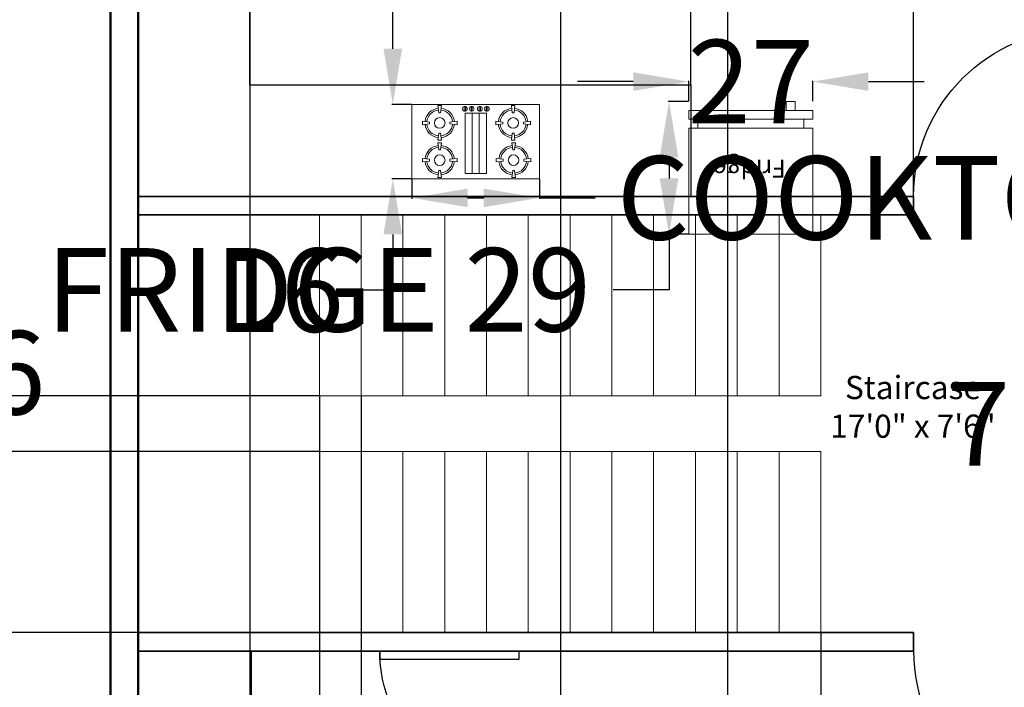
# Model space of a CAD drawing. Units: inches. Extents: x -230 to 384, y -962 to -183.
# Tile 3 of 6: x -121 to 91, y -640 to -496. Entities that reach past the tile are written whole.
import ezdxf

# ---------------------------------------------------------------- set-up
doc = ezdxf.new("R2010")
doc.units = ezdxf.units.IN
for name, color, linetype, lineweight in [('A-ANNO-DIMS', 2, 'Continuous', 18), ('A-ANNO-TEXT', 7, 'Continuous', 18), ('A-AREA-IDEN', 7, 'Continuous', 18), ('A-DOOR', 3, 'Continuous', 25), ('A-EQPM', 4, 'Continuous', 18), ('A-FLOR-STRS', 7, 'Continuous', 18), ('Inner Wall', 5, 'Continuous', 35), ('Kitchen', 4, 'Continuous', 25), ('Outer Wall', 1, 'Continuous', 50)]:
    doc.layers.add(name, color=color, linetype=linetype, lineweight=lineweight)
doc.styles.get("Standard").update_dxf_attribs({"font": 'arial.ttf'})
doc.dimstyles.get("Standard").update_dxf_attribs({"dimtxt": 18, "dimasz": 12, "dimexe": 0.18, "dimexo": 0.0625, "dimgap": 0.09, "dimtad": 0, "dimtih": 1, "dimtoh": 1, "dimdec": 0, "dimzin": 0, "dimdsep": 46, "dimlunit": 3, "dimtxsty": 'Standard', "dimcen": 0.09, "dimadec": 0, "dimazin": 0, "dimtfac": 1, "dimtdec": 0, "dimtofl": 0, "dimtmove": 0, "dimatfit": 3, "dimfxl": 1, "dimtolj": 1, "dimtzin": 0, "dimarcsym": 0})

# ---------------------------------------------------------------- blocks, each defined once
blk = doc.blocks.new('*U4')
for p, q in [((0, 0), (0, -4)), ((36, 0), (36, -4))]:
    blk.add_line(p, q)
blk.add_lwpolyline([(0, 0), (0, 36), (1.75, 36), (1.75, 0)], close=True)
blk.add_arc((0, 0), 36, 0, 90)
blk = doc.blocks.new('*U6')
for p, q in [((0, 0), (0, -4)), ((30, 0), (30, -4))]:
    blk.add_line(p, q)
blk.add_lwpolyline([(0, 0), (0, 30), (1.75, 30), (1.75, 0)], close=True)
blk.add_arc((0, 0), 30, 0, 90)
blk = doc.blocks.new('A$C57CF26DA')
for p, q in [((0, 0), (0, 420)), ((720, 420), (0, 420)), ((166.9, 413), (146.9, 413)), ((146.9, 413), (151.9, 373)), ((161.9, 373), (166.9, 413)), ((300, 390.9), (300, 49.1)), ((300, 390.9), (420, 390.9)), ((340, 390.9), (340, 49.1)), ((380, 390.9), (380, 49.1)), ((420, 390.9), (420, 49.1)), ((583.6, 413), (563.6, 413)), ((563.6, 413), (568.6, 373)), ((578.6, 373), (583.6, 413)), ((720, 0), (720, 420)), ((151.9, 373), (161.9, 373)), ((568.6, 373), (578.6, 373)), ((98.9, 320), (58.9, 325)), ((58.9, 325), (58.9, 305)), ((58.9, 305), (98.9, 310)), ((98.9, 310), (98.9, 320)), ((254.8, 325), (214.8, 320)), ((214.8, 320), (214.8, 310)), ((214.8, 310), (254.8, 305)), ((254.8, 305), (254.8, 325)), ((515.6, 320), (475.6, 325)), ((475.6, 325), (475.6, 305)), ((475.6, 305), (515.6, 310)), ((515.6, 310), (515.6, 320)), ((671.6, 325), (631.6, 320)), ((631.6, 320), (631.6, 310)), ((631.6, 310), (671.6, 305)), ((671.6, 305), (671.6, 325)), ((151.9, 257), (146.9, 217)), ((161.9, 257), (151.9, 257)), ((166.9, 217), (161.9, 257)), ((568.6, 257), (563.6, 217)), ((578.6, 257), (568.6, 257)), ((583.6, 217), (578.6, 257)), ((146.9, 217), (166.9, 217)), ((166.9, 203), (146.9, 203)), ((146.9, 203), (151.9, 163)), ((161.9, 163), (166.9, 203)), ((581.1, 203), (561.1, 203)), ((561.1, 203), (566.1, 163)), ((563.6, 217), (583.6, 217)), ((576.1, 163), (581.1, 203)), ((98.9, 110), (58.9, 115)), ((58.9, 115), (58.9, 95)), ((151.9, 163), (161.9, 163)), ((254.8, 115), (214.8, 110)), ((254.8, 95), (254.8, 115)), ((513.1, 110), (473.1, 115)), ((473.1, 115), (473.1, 95)), ((566.1, 163), (576.1, 163)), ((669, 115), (629, 110)), ((669, 95), (669, 115)), ((58.9, 95), (98.9, 100)), ((98.9, 100), (98.9, 110)), ((214.8, 110), (214.8, 100)), ((214.8, 100), (254.8, 95)), ((473.1, 95), (513.1, 100)), ((513.1, 100), (513.1, 110)), ((629, 110), (629, 100)), ((629, 100), (669, 95)), ((151.9, 47), (146.9, 7)), ((146.9, 7), (166.9, 7)), ((161.9, 47), (151.9, 47)), ((166.9, 7), (161.9, 47)), ((301.5, 38.7), (294.7, 38.7)), ((294.7, 38.7), (294.7, 11.3)), ((294.7, 11.3), (301.5, 11.3)), ((420, 49.1), (300, 49.1)), ((301.5, 11.3), (301.5, 38.7)), ((340.5, 38.7), (333.7, 38.7)), ((333.7, 38.7), (333.7, 11.3)), ((333.7, 11.3), (340.5, 11.3)), ((340.5, 11.3), (340.5, 38.7)), ((379.7, 11.3), (379.7, 38.7)), ((379.7, 38.7), (386.5, 38.7)), ((386.5, 11.3), (379.7, 11.3)), ((386.5, 38.7), (386.5, 11.3)), ((418.7, 11.3), (418.7, 38.7)), ((418.7, 38.7), (425.5, 38.7)), ((425.5, 11.3), (418.7, 11.3)), ((425.5, 38.7), (425.5, 11.3)), ((566.1, 47), (561.1, 7)), ((561.1, 7), (581.1, 7)), ((576.1, 47), (566.1, 47)), ((581.1, 7), (576.1, 47)), ((720, 0), (0, 0))]:
    blk.add_line(p, q)
for centre in [(156.9, 315), (573.6, 315), (156.9, 105), (571.1, 105)]:
    blk.add_circle(centre, 30)
for centre, radius, start, end in [((156.9, 315), 83, 95.5849, 174.4151), ((156.9, 315), 83, 5.5849, 84.4151), ((573.6, 315), 83, 95.5849, 174.4151), ((573.6, 315), 83, 5.5849, 84.4151), ((156.9, 315), 73, 95.3738, 174.6262), ((156.9, 315), 73, 5.3738, 84.6262), ((573.6, 315), 73, 95.3738, 174.6262), ((573.6, 315), 73, 5.3738, 84.6262), ((156.9, 315), 83, 185.5849, 264.4151), ((156.9, 315), 73, 185.3738, 264.6262), ((156.9, 315), 73, 275.3738, 354.6262), ((156.9, 315), 83, 275.5849, 354.4151), ((573.6, 315), 83, 185.5849, 264.4151), ((573.6, 315), 73, 185.3738, 264.6262), ((573.6, 315), 73, 275.3738, 354.6262), ((573.6, 315), 83, 275.5849, 354.4151), ((156.9, 105), 83, 95.5849, 174.4151), ((156.9, 105), 73, 95.3738, 174.6262), ((156.9, 105), 73, 5.3738, 84.6262), ((156.9, 105), 83, 5.5849, 84.4151), ((571.1, 105), 83, 95.5849, 174.4151), ((571.1, 105), 73, 95.3738, 174.6262), ((571.1, 105), 73, 5.3738, 84.6262), ((571.1, 105), 83, 5.5849, 84.4151), ((156.9, 105), 83, 185.5849, 264.4151), ((156.9, 105), 73, 185.3738, 264.6262), ((156.9, 105), 73, 275.3738, 354.6262), ((156.9, 105), 83, 275.5849, 354.4151), ((571.1, 105), 83, 185.5849, 264.4151), ((571.1, 105), 73, 185.3738, 264.6262), ((571.1, 105), 73, 275.3738, 354.6262), ((571.1, 105), 83, 275.5849, 354.4151), ((298.1, 25), 13.7, 104.4775, 255.5225), ((298.1, 25), 13.7, 284.4775, 75.5225), ((337.1, 25), 13.7, 104.4775, 255.5225), ((337.1, 25), 13.7, 284.4775, 75.5225), ((383.1, 25), 13.7, 104.4775, 255.5225), ((383.1, 25), 13.7, 284.4775, 75.5225), ((422.1, 25), 13.7, 104.4775, 255.5225), ((422.1, 25), 13.7, 284.4775, 75.5225)]:
    blk.add_arc(centre, radius, start, end)
blk = doc.blocks.new('REFRI-00')
for points in [[(-0.35, 0.35), (-0.35, -0.25), (0.35, -0.25), (0.35, 0.35), (-0.35, 0.35)], [(-0.3, -0.3), (-0.3, -0.25)], [(0.3, -0.3), (0.3, -0.25)], [(-0.35, -0.3), (-0.35, -0.35), (0.35, -0.35), (0.35, -0.3), (-0.35, -0.3)], [(-0.25, -0.35), (-0.25, -0.4), (-0.2, -0.4), (-0.2, -0.35)]]:
    blk.add_lwpolyline(points)
blk = doc.blocks.new('*D21')
at = {"layer": 'A-ANNO-DIMS', "color": 0, "lineweight": -2, "transparency": 16777216}
for p, q in [((-24.45, -424.96), (-24.45, -412.96)), ((-26.91, -436.96), (-24.27, -436.96)), ((-26.91, -450.25), (-24.27, -450.25)), ((-24.45, -462.25), (-24.45, -474.25)), ((-24.45, -474.25), (-36.45, -474.25))]:
    blk.add_line(p, q, dxfattribs=at)
at = {"layer": 'A-ANNO-DIMS', "color": 0, "transparency": 16777216}
for points in [[(-26.45, -424.96), (-22.45, -424.96), (-24.45, -436.96)], [(-26.45, -462.25), (-22.45, -462.25), (-24.45, -450.25)]]:
    blk.add_solid(points, dxfattribs=at)
at = {"layer": 'Defpoints', "color": 0, "transparency": 16777216}
for p in [(-26.97, -436.96), (-26.97, -450.25), (-24.45, -450.25)]:
    blk.add_point(p, dxfattribs=at)
at = {"layer": 'A-ANNO-DIMS', "color": 0, "transparency": 16777216, "insert": (-79.51, -474.25), "char_height": 18, "attachment_point": 5}
blk.add_mtext('\\A1;13 TYP.', dxfattribs=at)
blk = doc.blocks.new('*D23')
at = {"layer": 'A-ANNO-DIMS', "color": 0, "lineweight": -2, "transparency": 16777216}
for p, q in [((175.8, -568.08), (175.8, -583.43)), ((253.63, -568.08), (253.63, -583.43)), ((175.8, -583.25), (163.8, -583.25)), ((241.63, -583.25), (187.8, -583.25))]:
    blk.add_line(p, q, dxfattribs=at)
at = {"layer": 'A-ANNO-DIMS', "color": 0, "transparency": 16777216}
for points in [[(187.8, -581.25), (187.8, -585.25), (175.8, -583.25)], [(241.63, -581.25), (241.63, -585.25), (253.63, -583.25)]]:
    blk.add_solid(points, dxfattribs=at)
at = {"layer": 'Defpoints', "color": 0, "transparency": 16777216}
for p in [(175.8, -568.02), (253.63, -568.02), (175.8, -583.25)]:
    blk.add_point(p, dxfattribs=at)
at = {"layer": 'A-ANNO-DIMS', "color": 0, "transparency": 16777216, "insert": (119.97, -583.25), "char_height": 18, "attachment_point": 5}
blk.add_mtext('\\A1;78 TYP.', dxfattribs=at)
blk = doc.blocks.new('*D24')
at = {"layer": 'A-ANNO-DIMS', "color": 0, "lineweight": -2, "transparency": 16777216}
for p, q in [((14.93, -465.69), (14.93, -476.78)), ((88.09, -465.69), (88.09, -476.78)), ((26.93, -476.6), (76.09, -476.6)), ((88.09, -476.6), (100.09, -476.6))]:
    blk.add_line(p, q, dxfattribs=at)
at = {"layer": 'A-ANNO-DIMS', "color": 0, "transparency": 16777216}
for points in [[(26.93, -474.6), (26.93, -478.6), (14.93, -476.6)], [(76.09, -474.6), (76.09, -478.6), (88.09, -476.6)]]:
    blk.add_solid(points, dxfattribs=at)
at = {"layer": 'Defpoints', "color": 0, "transparency": 16777216}
for p in [(14.93, -465.63), (88.09, -465.63), (88.09, -476.6)]:
    blk.add_point(p, dxfattribs=at)
at = {"layer": 'A-ANNO-DIMS', "color": 0, "transparency": 16777216, "insert": (218.98, -476.6), "char_height": 18, "attachment_point": 5}
blk.add_mtext('\\A1;DINING SET 73 TYP.', dxfattribs=at)
blk = doc.blocks.new('*D28')
at = {"layer": 'A-ANNO-DIMS', "color": 0, "lineweight": -2, "transparency": 16777216}
for p, q in [((-36.67, -530.52), (-36.67, -534.76)), ((-9.19, -530.52), (-9.19, -534.76)), ((-24.67, -534.58), (-21.19, -534.58)), ((-9.19, -534.58), (2.81, -534.58))]:
    blk.add_line(p, q, dxfattribs=at)
at = {"layer": 'A-ANNO-DIMS', "color": 0, "transparency": 16777216}
for points in [[(-24.67, -532.58), (-24.67, -536.58), (-36.67, -534.58)], [(-21.19, -532.58), (-21.19, -536.58), (-9.19, -534.58)]]:
    blk.add_solid(points, dxfattribs=at)
at = {"layer": 'Defpoints', "color": 0, "transparency": 16777216}
for p in [(-36.67, -530.46), (-9.19, -530.46), (-9.19, -534.58)]:
    blk.add_point(p, dxfattribs=at)
at = {"layer": 'A-ANNO-DIMS', "color": 0, "transparency": 16777216, "insert": (82.05, -534.58), "char_height": 18, "attachment_point": 5}
blk.add_mtext('\\A1;COOKTOP 27', dxfattribs=at)
blk = doc.blocks.new('*D29')
at = {"layer": 'A-ANNO-DIMS', "color": 0, "lineweight": -2, "transparency": 16777216}
for p, q in [((-40.79, -502.43), (-40.79, -490.43)), ((-36.73, -514.43), (-40.97, -514.43)), ((-36.73, -530.46), (-40.97, -530.46)), ((-40.79, -542.46), (-40.79, -554.46)), ((-40.79, -554.46), (-52.79, -554.46))]:
    blk.add_line(p, q, dxfattribs=at)
at = {"layer": 'A-ANNO-DIMS', "color": 0, "transparency": 16777216}
for points in [[(-42.79, -502.43), (-38.79, -502.43), (-40.79, -514.43)], [(-42.79, -542.46), (-38.79, -542.46), (-40.79, -530.46)]]:
    blk.add_solid(points, dxfattribs=at)
at = {"layer": 'Defpoints', "color": 0, "transparency": 16777216}
for p in [(-36.67, -514.43), (-40.79, -530.46), (-36.67, -530.46)]:
    blk.add_point(p, dxfattribs=at)
at = {"layer": 'A-ANNO-DIMS', "color": 0, "transparency": 16777216, "insert": (-64.92, -554.46), "char_height": 18, "attachment_point": 5}
blk.add_mtext('\\A1;16', dxfattribs=at)
blk = doc.blocks.new('*D30')
at = {"layer": 'A-ANNO-DIMS', "color": 0, "lineweight": -2, "transparency": 16777216}
for p, q in [((22.93, -513.82), (18.53, -513.82)), ((18.71, -525.82), (18.71, -530.39)), ((22.93, -542.39), (18.53, -542.39)), ((18.71, -542.39), (18.71, -554.39)), ((18.71, -554.39), (6.71, -554.39))]:
    blk.add_line(p, q, dxfattribs=at)
at = {"layer": 'A-ANNO-DIMS', "color": 0, "transparency": 16777216}
for points in [[(16.71, -525.82), (20.71, -525.82), (18.71, -513.82)], [(16.71, -530.39), (20.71, -530.39), (18.71, -542.39)]]:
    blk.add_solid(points, dxfattribs=at)
at = {"layer": 'Defpoints', "color": 0, "transparency": 16777216}
for p in [(22.99, -513.82), (18.71, -542.39), (22.99, -542.39)]:
    blk.add_point(p, dxfattribs=at)
at = {"layer": 'A-ANNO-DIMS', "color": 0, "transparency": 16777216, "insert": (-56.78, -554.39), "char_height": 18, "attachment_point": 5}
blk.add_mtext('\\A1;FRIDGE 29', dxfattribs=at)
blk = doc.blocks.new('*D31')
at = {"layer": 'A-ANNO-DIMS', "color": 0, "lineweight": -2, "transparency": 16777216}
for p, q in [((10.99, -509.53), (-1.01, -509.53)), ((22.99, -513.76), (22.99, -509.35)), ((49.66, -513.76), (49.66, -509.35)), ((61.66, -509.53), (73.66, -509.53))]:
    blk.add_line(p, q, dxfattribs=at)
at = {"layer": 'A-ANNO-DIMS', "color": 0, "transparency": 16777216}
for points in [[(10.99, -507.53), (10.99, -511.53), (22.99, -509.53)], [(61.66, -507.53), (61.66, -511.53), (49.66, -509.53)]]:
    blk.add_solid(points, dxfattribs=at)
at = {"layer": 'Defpoints', "color": 0, "transparency": 16777216}
for p in [(22.99, -509.53), (22.99, -513.82), (49.66, -513.82)]:
    blk.add_point(p, dxfattribs=at)
at = {"layer": 'A-ANNO-DIMS', "color": 0, "transparency": 16777216, "insert": (36.33, -509.53), "char_height": 18, "attachment_point": 5}
blk.add_mtext('\\A1;27', dxfattribs=at)
blk = doc.blocks.new('*D33')
at = {"layer": 'A-ANNO-DIMS', "color": 0, "lineweight": -2, "transparency": 16777216}
for p, q in [((-101.66, -229.25), (-136.23, -229.25)), ((-136.05, -241.25), (-136.05, -562.97)), ((-136.05, -903.25), (-136.05, -581.53)), ((-101.66, -915.25), (-136.23, -915.25))]:
    blk.add_line(p, q, dxfattribs=at)
at = {"layer": 'A-ANNO-DIMS', "color": 0, "transparency": 16777216}
for points in [[(-138.05, -241.25), (-134.05, -241.25), (-136.05, -229.25)], [(-138.05, -903.25), (-134.05, -903.25), (-136.05, -915.25)]]:
    blk.add_solid(points, dxfattribs=at)
at = {"layer": 'Defpoints', "color": 0, "transparency": 16777216}
for p in [(-101.6, -229.25), (-136.05, -915.25), (-101.6, -915.25)]:
    blk.add_point(p, dxfattribs=at)
at = {"layer": 'A-ANNO-DIMS', "color": 0, "transparency": 16777216, "insert": (-136.05, -572.25), "char_height": 18, "attachment_point": 5}
blk.add_mtext('\\A1;686', dxfattribs=at)
blk = doc.blocks.new('*D38')
at = {"layer": 'A-ANNO-DIMS', "color": 0, "lineweight": -2, "transparency": 16777216}
for p, q in [((-56.6, -628.32), (-56.6, -949.88)), ((51.4, -628.32), (51.4, -949.88)), ((-44.6, -949.7), (-21.75, -949.7)), ((39.4, -949.7), (16.54, -949.7))]:
    blk.add_line(p, q, dxfattribs=at)
at = {"layer": 'A-ANNO-DIMS', "color": 0, "transparency": 16777216}
for points in [[(-44.6, -947.7), (-44.6, -951.7), (-56.6, -949.7)], [(39.4, -947.7), (39.4, -951.7), (51.4, -949.7)]]:
    blk.add_solid(points, dxfattribs=at)
at = {"layer": 'Defpoints', "color": 0, "transparency": 16777216}
for p in [(-56.6, -628.25), (51.4, -628.25), (51.4, -949.7)]:
    blk.add_point(p, dxfattribs=at)
at = {"layer": 'A-ANNO-DIMS', "color": 0, "transparency": 16777216, "insert": (-2.6, -949.7), "char_height": 18, "attachment_point": 5}
blk.add_mtext('\\A1;108', dxfattribs=at)
blk = doc.blocks.new('*D39')
at = {"layer": 'A-ANNO-DIMS', "color": 0, "lineweight": -2, "transparency": 16777216}
for p, q in [((-56.66, -589.25), (-136.23, -589.25)), ((-136.05, -601.25), (-136.05, -616.25)), ((-56.66, -628.25), (-136.23, -628.25)), ((-136.05, -628.25), (-136.05, -640.25)), ((-136.05, -640.25), (-148.05, -640.25))]:
    blk.add_line(p, q, dxfattribs=at)
at = {"layer": 'A-ANNO-DIMS', "color": 0, "transparency": 16777216}
for points in [[(-138.05, -601.25), (-134.05, -601.25), (-136.05, -589.25)], [(-138.05, -616.25), (-134.05, -616.25), (-136.05, -628.25)]]:
    blk.add_solid(points, dxfattribs=at)
at = {"layer": 'Defpoints', "color": 0, "transparency": 16777216}
for p in [(-56.6, -589.25), (-136.05, -628.25), (-56.6, -628.25)]:
    blk.add_point(p, dxfattribs=at)
at = {"layer": 'A-ANNO-DIMS', "color": 0, "transparency": 16777216, "insert": (-161.05, -640.25), "char_height": 18, "attachment_point": 5}
blk.add_mtext('\\A1;39', dxfattribs=at)
blk = doc.blocks.new('*D41')
at = {"layer": 'A-ANNO-DIMS', "color": 0, "lineweight": -2, "transparency": 16777216}
for p, q in [((-95.6, -454.32), (-95.6, -949.88)), ((-71.6, -454.32), (-71.6, -949.88)), ((-107.6, -949.7), (-119.6, -949.7)), ((-59.6, -949.7), (-47.6, -949.7))]:
    blk.add_line(p, q, dxfattribs=at)
at = {"layer": 'A-ANNO-DIMS', "color": 0, "transparency": 16777216}
for points in [[(-107.6, -947.7), (-107.6, -951.7), (-95.6, -949.7)], [(-59.6, -947.7), (-59.6, -951.7), (-71.6, -949.7)]]:
    blk.add_solid(points, dxfattribs=at)
at = {"layer": 'Defpoints', "color": 0, "transparency": 16777216}
for p in [(-95.6, -454.25), (-71.6, -454.25), (-71.6, -949.7)]:
    blk.add_point(p, dxfattribs=at)
at = {"layer": 'A-ANNO-DIMS', "color": 0, "transparency": 16777216, "insert": (-34.5, -949.7), "char_height": 18, "attachment_point": 5}
blk.add_mtext('\\A1;24', dxfattribs=at)
blk = doc.blocks.new('*D43')
at = {"layer": 'A-ANNO-DIMS', "color": 0, "lineweight": -2, "transparency": 16777216}
for p, q in [((-71.6, -510.19), (-71.6, -194.62)), ((-59.6, -194.8), (-37.15, -194.8)), ((11.4, -194.8), (-11.05, -194.8)), ((23.4, -510.19), (23.4, -194.62))]:
    blk.add_line(p, q, dxfattribs=at)
at = {"layer": 'A-ANNO-DIMS', "color": 0, "transparency": 16777216}
for points in [[(-59.6, -192.8), (-59.6, -196.8), (-71.6, -194.8)], [(11.4, -192.8), (11.4, -196.8), (23.4, -194.8)]]:
    blk.add_solid(points, dxfattribs=at)
at = {"layer": 'Defpoints', "color": 0, "transparency": 16777216}
for p in [(23.4, -194.8), (-71.6, -510.25), (23.4, -510.25)]:
    blk.add_point(p, dxfattribs=at)
at = {"layer": 'A-ANNO-DIMS', "color": 0, "transparency": 16777216, "insert": (-24.1, -194.8), "char_height": 18, "attachment_point": 5}
blk.add_mtext('\\A1;95', dxfattribs=at)
blk = doc.blocks.new('*D46')
at = {"layer": 'A-ANNO-DIMS', "color": 0, "lineweight": -2, "transparency": 16777216}
for p, q in [((-56.6, -577.32), (-56.6, -949.88)), ((-47.6, -577.32), (-47.6, -949.88)), ((-68.6, -949.7), (-80.6, -949.7)), ((-35.6, -949.7), (-23.6, -949.7))]:
    blk.add_line(p, q, dxfattribs=at)
at = {"layer": 'A-ANNO-DIMS', "color": 0, "transparency": 16777216}
for points in [[(-68.6, -947.7), (-68.6, -951.7), (-56.6, -949.7)], [(-35.6, -947.7), (-35.6, -951.7), (-47.6, -949.7)]]:
    blk.add_solid(points, dxfattribs=at)
at = {"layer": 'Defpoints', "color": 0, "transparency": 16777216}
for p in [(-56.6, -577.25), (-47.6, -577.25), (-47.6, -949.7)]:
    blk.add_point(p, dxfattribs=at)
at = {"layer": 'A-ANNO-DIMS', "color": 0, "transparency": 16777216, "insert": (-17.59, -949.7), "char_height": 18, "attachment_point": 5}
blk.add_mtext('\\A1;9', dxfattribs=at)
blk = doc.blocks.new('*D47')
at = {"layer": 'A-ANNO-DIMS', "color": 0, "lineweight": -2, "transparency": 16777216}
for p, q in [((-95.60199, -628.31695), (-95.60199, -949.88445)), ((-56.60199, -628.31695), (-56.60199, -949.88445)), ((-107.60199, -949.70445), (-119.60199, -949.70445)), ((-44.60199, -949.70445), (-32.60199, -949.70445))]:
    blk.add_line(p, q, dxfattribs=at)
at = {"layer": 'A-ANNO-DIMS', "color": 0, "transparency": 16777216}
for points in [[(-107.60199, -947.70445), (-107.60199, -951.70445), (-95.60199, -949.70445)], [(-44.60199, -947.70445), (-44.60199, -951.70445), (-56.60199, -949.70445)]]:
    blk.add_solid(points, dxfattribs=at)
at = {"layer": 'Defpoints', "color": 0, "transparency": 16777216}
for p in [(-95.60199, -628.25445), (-56.60199, -628.25445), (-56.60199, -949.70445)]:
    blk.add_point(p, dxfattribs=at)
at = {"layer": 'A-ANNO-DIMS', "color": 0, "transparency": 16777216, "insert": (-76.10199, -949.70445), "char_height": 18, "attachment_point": 5}
blk.add_mtext('\\A1;39', dxfattribs=at)
blk = doc.blocks.new('*D48')
at = {"layer": 'A-ANNO-DIMS', "color": 0, "lineweight": -2, "transparency": 16777216}
for p, q in [((-136.05, -565.25), (-136.05, -553.25)), ((-56.66, -577.25), (-136.23, -577.25)), ((-56.66, -589.25), (-136.23, -589.25)), ((-136.05, -601.25), (-136.05, -613.25)), ((-136.05, -613.25), (-148.05, -613.25))]:
    blk.add_line(p, q, dxfattribs=at)
at = {"layer": 'A-ANNO-DIMS', "color": 0, "transparency": 16777216}
for points in [[(-138.05, -565.25), (-134.05, -565.25), (-136.05, -577.25)], [(-138.05, -601.25), (-134.05, -601.25), (-136.05, -589.25)]]:
    blk.add_solid(points, dxfattribs=at)
at = {"layer": 'Defpoints', "color": 0, "transparency": 16777216}
for p in [(-56.6, -577.25), (-136.05, -589.25), (-56.6, -589.25)]:
    blk.add_point(p, dxfattribs=at)
at = {"layer": 'A-ANNO-DIMS', "color": 0, "transparency": 16777216, "insert": (-160.09, -613.25), "char_height": 18, "attachment_point": 5}
blk.add_mtext('\\A1;12', dxfattribs=at)
blk = doc.blocks.new('*D50')
at = {"layer": 'A-ANNO-DIMS', "color": 0, "lineweight": -2, "transparency": 16777216}
for p, q in [((59.39801, -194.80445), (47.39801, -194.80445)), ((71.39801, -534.19195), (71.39801, -194.62445)), ((107.39801, -534.19195), (107.39801, -194.62445)), ((119.39801, -194.80445), (131.39801, -194.80445))]:
    blk.add_line(p, q, dxfattribs=at)
at = {"layer": 'A-ANNO-DIMS', "color": 0, "transparency": 16777216}
for points in [[(59.39801, -192.80445), (59.39801, -196.80445), (71.39801, -194.80445)], [(119.39801, -192.80445), (119.39801, -196.80445), (107.39801, -194.80445)]]:
    blk.add_solid(points, dxfattribs=at)
at = {"layer": 'Defpoints', "color": 0, "transparency": 16777216}
for p in [(107.39801, -194.80445), (71.39801, -534.25445), (107.39801, -534.25445)]:
    blk.add_point(p, dxfattribs=at)
at = {"layer": 'A-ANNO-DIMS', "color": 0, "transparency": 16777216, "insert": (89.39801, -194.80445), "char_height": 18, "attachment_point": 5}
blk.add_mtext('\\A1;36', dxfattribs=at)
blk = doc.blocks.new('*D51')
at = {"layer": 'A-ANNO-DIMS', "color": 0, "lineweight": -2, "transparency": 16777216}
for p, q in [((-16.60199, -194.80445), (-28.60199, -194.80445)), ((-4.60199, -875.19195), (-4.60199, -194.62445)), ((31.39801, -875.19195), (31.39801, -194.62445)), ((43.39801, -194.80445), (55.39801, -194.80445))]:
    blk.add_line(p, q, dxfattribs=at)
at = {"layer": 'A-ANNO-DIMS', "color": 0, "transparency": 16777216}
for points in [[(-16.60199, -192.80445), (-16.60199, -196.80445), (-4.60199, -194.80445)], [(43.39801, -192.80445), (43.39801, -196.80445), (31.39801, -194.80445)]]:
    blk.add_solid(points, dxfattribs=at)
at = {"layer": 'Defpoints', "color": 0, "transparency": 16777216}
for p in [(31.39801, -194.80445), (-4.60199, -875.25445), (31.39801, -875.25445)]:
    blk.add_point(p, dxfattribs=at)
at = {"layer": 'A-ANNO-DIMS', "color": 0, "transparency": 16777216, "insert": (13.39801, -194.80445), "char_height": 18, "attachment_point": 5}
blk.add_mtext('\\A1;36', dxfattribs=at)

msp = doc.modelspace()

# ---------------------------------------------------------------- linework, layer by layer
at = {"layer": 'A-FLOR-STRS'}
for p, q in [((-56.6, -628.25), (-56.6, -538.25)), ((-47.6, -577.25), (-47.6, -538.25)), ((-38.6, -577.25), (-38.6, -538.25)), ((-29.6, -577.25), (-29.6, -538.25)), ((-20.6, -577.25), (-20.6, -538.25)), ((-11.6, -577.25), (-11.6, -538.25)), ((-2.6, -577.25), (-2.6, -538.25)), ((6.4, -577.25), (6.4, -538.25)), ((15.4, -577.25), (15.4, -538.25)), ((24.4, -577.25), (24.4, -538.25)), ((33.4, -577.25), (33.4, -538.25)), ((42.4, -577.25), (42.4, -538.25)), ((51.4, -577.25), (51.4, -538.25)), ((-56.6, -577.25), (51.4, -577.25)), ((-56.6, -589.25), (51.4, -589.25)), ((-47.6, -628.25), (-47.6, -589.25)), ((-38.6, -628.25), (-38.6, -589.25)), ((-29.6, -628.25), (-29.6, -589.25)), ((-20.6, -628.25), (-20.6, -589.25)), ((-11.6, -628.25), (-11.6, -589.25)), ((-2.6, -628.25), (-2.6, -589.25)), ((6.4, -628.25), (6.4, -589.25)), ((15.4, -628.25), (15.4, -589.25)), ((24.4, -628.25), (24.4, -589.25)), ((33.4, -628.25), (33.4, -589.25)), ((42.4, -628.25), (42.4, -589.25)), ((51.4, -628.25), (51.4, -589.25))]:
    msp.add_line(p, q, dxfattribs=at)
at = {"layer": 'Inner Wall'}
for p, q in [((-95.6, -534.25), (71.4, -534.25)), ((71.4, -534.25), (71.4, -538.25)), ((-95.6, -538.25), (71.4, -538.25)), ((-95.6, -628.25), (71.4, -628.25)), ((71.4, -628.25), (71.4, -632.25)), ((-95.6, -632.25), (71.4, -632.25))]:
    msp.add_line(p, q, dxfattribs=at)
at = {"layer": 'Kitchen'}
for p, q in [((-71.6, -510.25), (-71.6, -454.25)), ((-71.6, -510.25), (23.4, -510.25)), ((23.4, -510.25), (23.4, -534.25))]:
    msp.add_line(p, q, dxfattribs=at)
msp.add_lwpolyline([(-95.6, -632.25), (-71.3, -632.25), (-71.3, -693.25), (-95.6, -693.25)], close=True, dxfattribs=at)
at = {"layer": 'Outer Wall'}
msp.add_line((-95.6, -909.25), (-95.6, -235.25), dxfattribs=at)
msp.add_lwpolyline([(272.4, -915.25), (-101.6, -915.25), (-101.6, -229.25), (272.4, -229.25)], close=True, dxfattribs=at)

# ---------------------------------------------------------------- block references
at = {"layer": 'A-DOOR', "xscale": -1}
msp.add_blockref('*U4', (107.4, -534.25), dxfattribs=at)
at = {"layer": 'A-DOOR', "rotation": 180}
msp.add_blockref('*U4', (107.4, -632.25), dxfattribs=at)
at = {"layer": 'A-DOOR', "xscale": -1, "rotation": 90}
msp.add_blockref('*U6', (-13.6, -632.25), dxfattribs=at)
at = {"layer": 'A-EQPM', "rotation": 180}
for name, p, xscale, yscale, zscale in [('A$C57CF26DA', (-36.67, -514.43), -0.0381707681172169, 0.0381707681172169, 0.0381707681172169), ('REFRI-00', (36.33, -529.06), 38.0932829071003, 38.0932829071003, 38.0932829071003)]:
    msp.add_blockref(name, p, dxfattribs=dict(at, xscale=xscale, yscale=yscale, zscale=zscale))

# ---------------------------------------------------------------- texts
at = {"layer": 'A-ANNO-TEXT', "insert": (45, -530.24), "char_height": 3.878, "attachment_point": 1, "rotation": 180}
msp.add_mtext_dynamic_manual_height_columns('\\pxqc;{\\fTimes New Roman|b0|i0|c0|p18;Fridge}', width=17.9518, gutter_width=4.85, heights=[0], dxfattribs=at)
at = {"layer": 'A-AREA-IDEN', "insert": (95.8, -572.94), "char_height": 5, "attachment_point": 3}
msp.add_mtext_dynamic_manual_height_columns('\\pxqc;{\\fTimes New Roman|b0|i0|c0|p18;Staircase\\P17\'0" x 7\'6"}', width=49.1019, gutter_width=12.5, heights=[0], dxfattribs=at)

# ---------------------------------------------------------------- dimensions: what is measured, and where the dimension line sits
at = {"layer": 'A-ANNO-DIMS'}
for base, p1, p2, picture, middle in [((23.4, -194.8), (-71.6, -510.25), (23.4, -510.25), '*D43', (-24.1, -194.8)), ((31.4, -194.8), (-4.6, -875.25), (31.4, -875.25), '*D51', (13.4, -194.8)), ((107.4, -194.8), (71.4, -534.25), (107.4, -534.25), '*D50', (89.4, -194.8)), ((-71.6, -949.7), (-95.6, -454.25), (-71.6, -454.25), '*D41', (-34.5, -949.7)), ((-47.6, -949.7), (-56.6, -577.25), (-47.6, -577.25), '*D46', (-17.59, -949.7)), ((-56.6, -949.7), (-95.6, -628.25), (-56.6, -628.25), '*D47', (-76.1, -949.7)), ((51.4, -949.7), (-56.6, -628.25), (51.4, -628.25), '*D38', (-2.6, -949.7))]:
    dim = msp.add_linear_dim(base=base, p1=p1, p2=p2, dimstyle='Standard', override={"dimdec": 0, "dimlfac": 1, "dimrnd": 0, "dimzin": 0, "dimdsep": 46, "dimlunit": 2}, dxfattribs=at)
    dim.commit()
    dim.dimension.update_dxf_attribs({"geometry": picture, "text_midpoint": middle})
for base, p1, p2, angle, picture, middle in [((-136.05, -915.25), (-101.6, -229.25), (-101.6, -915.25), 90, '*D33', (-136.05, -572.25)), ((-40.79, -530.46), (-36.67, -514.43), (-36.67, -530.46), 270, '*D29', (-64.92, -554.46)), ((22.99, -509.53), (49.66, -513.82), (22.99, -513.82), 180, '*D31', (36.33, -509.53)), ((-136.05, -589.25), (-56.6, -577.25), (-56.6, -589.25), 90, '*D48', (-160.09, -613.25)), ((-136.05, -628.25), (-56.6, -589.25), (-56.6, -628.25), 90, '*D39', (-161.05, -640.25))]:
    dim = msp.add_linear_dim(base=base, p1=p1, p2=p2, angle=angle, dimstyle='Standard', override={"dimdec": 0, "dimlfac": 1, "dimrnd": 0, "dimzin": 0, "dimdsep": 46, "dimlunit": 2}, dxfattribs=at)
    dim.commit()
    dim.dimension.update_dxf_attribs({"geometry": picture, "text_midpoint": middle})
for base, p1, p2, angle, text, picture, middle in [((-24.45, -450.25), (-26.97, -436.96), (-26.97, -450.25), 270, '<> TYP.', '*D21', (-79.51, -474.25)), ((18.71, -542.39), (22.99, -513.82), (22.99, -542.39), 270, 'FRIDGE <>', '*D30', (-56.78, -554.39)), ((175.8, -583.25), (253.63, -568.02), (175.8, -568.02), 180, '<> TYP.', '*D23', (119.97, -583.25))]:
    dim = msp.add_linear_dim(base=base, p1=p1, p2=p2, angle=angle, text=text, dimstyle='Standard', override={"dimdec": 0, "dimlfac": 1, "dimrnd": 0, "dimzin": 0, "dimdsep": 46, "dimlunit": 2}, dxfattribs=at)
    dim.commit()
    dim.dimension.update_dxf_attribs({"geometry": picture, "text_midpoint": middle})
for base, p1, p2, text, picture, middle in [((88.09, -476.6), (14.93, -465.63), (88.09, -465.63), 'DINING SET <> TYP.', '*D24', (218.98, -476.6)), ((-9.19, -534.58), (-36.67, -530.46), (-9.19, -530.46), 'COOKTOP <>', '*D28', (82.05, -534.58))]:
    dim = msp.add_linear_dim(base=base, p1=p1, p2=p2, text=text, dimstyle='Standard', override={"dimdec": 0, "dimlfac": 1, "dimrnd": 0, "dimzin": 0, "dimdsep": 46, "dimlunit": 2}, dxfattribs=at)
    dim.commit()
    dim.dimension.update_dxf_attribs({"geometry": picture, "text_midpoint": middle})

doc.saveas('drawing.dxf')
